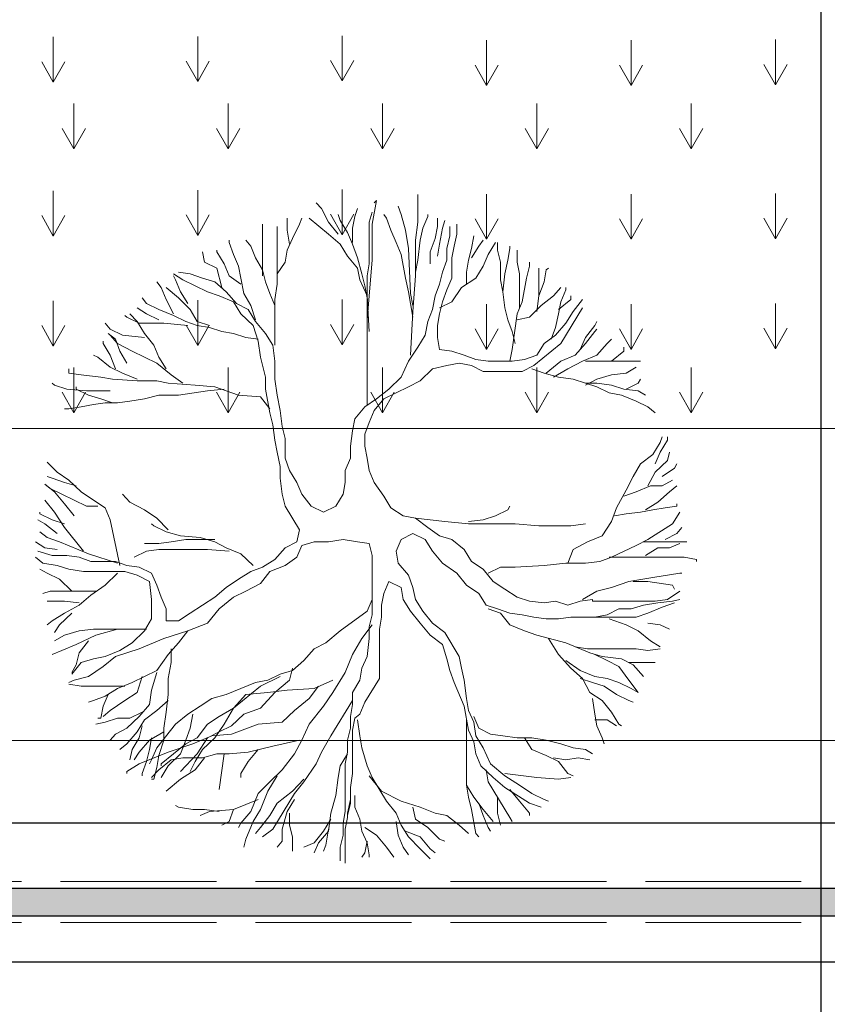
# Model space of a CAD drawing. Units: millimetres. Extents: x 595116 to 630915, y 909473 to 920225.
# Tile 42 of 134: x 629682 to 629744, y 919141 to 919216. Entities that reach past the tile are written whole.
import ezdxf

# ---------------------------------------------------------------- set-up
doc = ezdxf.new("R2010")
doc.units = ezdxf.units.MM
doc.linetypes.add('ACAD_ISO02W100', pattern=[15, 12, -3])
for name, color, linetype, lineweight in [('C-PROP', 7, 'Continuous', 25), ('C-PROP-REF', 240, 'ACAD_ISO02W100', 13), ('Dimension', 3, 'Continuous', 18), ('L-PLNT', 85, 'Continuous', 13)]:
    doc.layers.add(name, color=color, linetype=linetype, lineweight=lineweight)
doc.styles.get("Standard").update_dxf_attribs({"font": 'arial.ttf'})
doc.dimstyles.new('ISO-25', dxfattribs={"dimtxt": 9, "dimasz": 6, "dimexe": 1.25, "dimexo": 0.625, "dimtad": 1, "dimlunit": 4, "dimtxsty": 'Standard', "dimcen": 2.5, "dimadec": 0, "dimazin": 0, "dimtfac": 1, "dimtmove": 0, "dimatfit": 3, "dimfxl": 1, "dimarcsym": 0})

# ---------------------------------------------------------------- blocks, each defined once
blk = doc.blocks.new('A$C143125F4')
for p, q in [((2.1554, 4.9368), (2.1171, 4.9816)), ((2.5383, 4.8203), (2.5711, 4.9995)), ((2.5711, 4.9995), (2.5547, 4.9816)), ((2.883, 4.8338), (2.883, 5.0443)), ((2.2101, 4.8338), (2.1554, 4.9368)), ((2.407, 4.8786), (2.4289, 4.9368)), ((2.5164, 4.8338), (2.5383, 4.9099)), ((2.7571, 4.892), (2.7353, 4.9547)), ((1.8983, 4.7755), (1.8983, 4.8651)), ((1.9913, 4.8203), (2.0077, 4.8651)), ((2.2101, 4.7442), (2.0624, 4.8651)), ((2.2812, 4.7442), (2.2101, 4.8338)), ((2.2976, 4.8472), (2.2812, 4.892)), ((2.3523, 4.7576), (2.2976, 4.8472)), ((2.3906, 4.789), (2.407, 4.8786)), ((2.5164, 4.5202), (2.5164, 4.8338)), ((2.6477, 4.8651), (2.6259, 4.892)), ((2.6806, 4.7755), (2.6477, 4.8651)), ((2.79, 4.7755), (2.7571, 4.892)), ((2.8666, 4.6994), (2.883, 4.8338)), ((2.9213, 4.789), (2.9596, 4.8786)), ((2.9596, 4.8786), (2.9596, 4.892)), ((3.0307, 4.8024), (3.0307, 4.8651)), ((3.069, 4.789), (3.0854, 4.8472)), ((1.7123, 4.4306), (1.7123, 4.8203)), ((1.8217, 4.3679), (1.8217, 4.8024)), ((1.9147, 4.668), (1.8983, 4.7755)), ((1.9366, 4.7128), (1.9913, 4.8203)), ((2.3906, 4.668), (2.3523, 4.7576)), ((2.3906, 4.6814), (2.3906, 4.789)), ((2.5383, 4.5471), (2.5383, 4.8203)), ((2.7189, 4.6814), (2.6806, 4.7755)), ((2.8119, 4.6367), (2.79, 4.7755)), ((2.8994, 4.6994), (2.9213, 4.789)), ((3.0143, 4.7128), (3.0307, 4.8024)), ((3.0471, 4.668), (3.069, 4.789)), ((3.1237, 4.7307), (3.1237, 4.8024)), ((3.1784, 4.7442), (3.1784, 4.8203)), ((1.4606, 4.6814), (1.4606, 4.6994)), ((1.4935, 4.5919), (1.4606, 4.6814)), ((1.6247, 4.6546), (1.5865, 4.6994)), ((1.8983, 4.6232), (1.9366, 4.7128)), ((2.2976, 4.668), (2.2101, 4.7442)), ((2.7571, 4.5919), (2.7189, 4.6814)), ((2.8666, 4.4306), (2.8666, 4.6994)), ((2.883, 4.5471), (2.8994, 4.6994)), ((2.976, 4.6098), (3.0143, 4.7128)), ((3.1018, 4.6367), (3.1237, 4.7307)), ((3.1565, 4.6546), (3.1784, 4.7442)), ((3.2878, 4.6367), (3.3042, 4.7307)), ((3.3425, 4.6546), (3.3753, 4.6994)), ((3.4136, 4.5919), (3.4683, 4.6814)), ((3.4847, 4.6232), (3.4847, 4.6814)), ((1.2746, 4.5336), (1.2582, 4.6098)), ((1.3676, 4.6098), (1.3676, 4.6232)), ((1.4223, 4.5202), (1.3676, 4.6098)), ((1.6576, 4.565), (1.6247, 4.6546)), ((1.8819, 4.5336), (1.8983, 4.6232)), ((2.3523, 4.5784), (2.2976, 4.668)), ((2.4289, 4.565), (2.3906, 4.668)), ((2.8283, 4.2962), (2.8119, 4.6367)), ((2.976, 4.5202), (2.976, 4.6098)), ((3.0307, 4.5784), (3.0471, 4.668)), ((3.1018, 4.5471), (3.1018, 4.6367)), ((3.1401, 4.565), (3.1565, 4.6546)), ((3.2659, 4.5471), (3.2878, 4.6367)), ((3.2878, 4.565), (3.3425, 4.6546)), ((3.5066, 4.5336), (3.4847, 4.6232)), ((3.5613, 4.5471), (3.5777, 4.6367)), ((3.5777, 4.6367), (3.5777, 4.6546)), ((3.6324, 4.5336), (3.6324, 4.6232)), ((1.3676, 4.4888), (1.2746, 4.5336)), ((1.5317, 4.5023), (1.4935, 4.5919)), ((1.7123, 4.4754), (1.6576, 4.565)), ((1.8217, 4.444), (1.8819, 4.5336)), ((2.4289, 4.4888), (2.3523, 4.5784)), ((2.4617, 4.444), (2.4289, 4.565)), ((2.5, 4.0991), (2.5383, 4.5471)), ((2.79, 4.4127), (2.7571, 4.5919)), ((2.8666, 4.4575), (2.883, 4.5471)), ((3.069, 4.4575), (3.1018, 4.5471)), ((3.1401, 4.4127), (3.1401, 4.565)), ((3.2495, 4.4575), (3.2659, 4.5471)), ((3.3753, 4.5023), (3.4136, 4.5919)), ((3.5066, 4.3992), (3.5066, 4.5336)), ((3.5394, 4.444), (3.5613, 4.5471)), ((3.6488, 4.444), (3.6324, 4.5336)), ((3.7254, 4.5023), (3.7254, 4.5336)), ((1.0777, 4.4575), (1.1652, 4.444)), ((1.4059, 4.341), (1.3676, 4.4888)), ((1.4606, 4.4306), (1.4223, 4.5202)), ((1.5482, 4.4127), (1.5317, 4.5023)), ((1.7342, 4.3858), (1.7123, 4.4754)), ((2.4453, 4.3992), (2.4289, 4.4888)), ((2.5, 4.4306), (2.5164, 4.5202)), ((3.0471, 4.3679), (3.069, 4.4575)), ((3.2495, 4.3679), (3.2495, 4.4575)), ((3.3206, 4.4127), (3.3753, 4.5023)), ((3.7035, 4.4127), (3.7254, 4.5023)), ((3.7965, 4.2783), (3.7965, 4.4888)), ((3.8348, 4.3858), (3.8512, 4.4754)), ((3.8512, 4.4754), (3.8677, 4.4888)), ((0.9464, 4.341), (0.9136, 4.3858)), ((1.1105, 4.3992), (1.0394, 4.444)), ((1.0558, 4.3992), (1.0394, 4.4306)), ((1.0941, 4.3096), (1.0558, 4.3992)), ((1.2965, 4.3096), (1.1105, 4.3992)), ((1.1652, 4.444), (1.2582, 4.4127)), ((1.2582, 4.4127), (1.3512, 4.3858)), ((1.3512, 4.3858), (1.4387, 4.3096)), ((1.5482, 4.3679), (1.4606, 4.4306)), ((1.57, 4.2962), (1.5482, 4.4127)), ((1.767, 4.2962), (1.7342, 4.3858)), ((2.5, 4.2783), (2.4453, 4.3992)), ((2.4836, 4.3544), (2.4617, 4.444)), ((2.5, 3.4584), (2.5, 4.4306)), ((2.8119, 4.3096), (2.79, 4.4127)), ((2.8447, 4.1618), (2.8666, 4.4306)), ((3.1018, 4.3231), (3.1401, 4.4127)), ((3.2112, 4.341), (3.3206, 4.4127)), ((3.523, 4.3096), (3.5066, 4.3992)), ((3.523, 4.3096), (3.5394, 4.444)), ((3.6488, 4.1887), (3.6488, 4.444)), ((3.6707, 4.2335), (3.7035, 4.4127)), ((3.7965, 4.2783), (3.8348, 4.3858)), ((0.9847, 4.2514), (0.9464, 4.341)), ((1.0777, 4.2648), (0.9847, 4.341)), ((1.1488, 4.22), (1.0941, 4.3096)), ((1.384, 4.2783), (1.2965, 4.3096)), ((1.4387, 4.3096), (1.5153, 4.22)), ((1.8053, 4.2514), (1.8217, 4.3679)), ((2.5, 4.2648), (2.4836, 4.3544)), ((2.8283, 4.22), (2.8119, 4.3096)), ((3.0143, 4.2783), (3.0471, 4.3679)), ((3.069, 4.2335), (3.1018, 4.3231)), ((3.1401, 4.2335), (3.2112, 4.341)), ((3.5394, 4.1887), (3.523, 4.3096)), ((3.906, 4.2783), (3.9607, 4.341)), ((3.9607, 4.2335), (3.999, 4.3231)), ((3.999, 4.3231), (3.999, 4.341)), ((0.837, 4.22), (0.8042, 4.2648)), ((1.0394, 4.1439), (0.9847, 4.2514)), ((1.1652, 4.1752), (1.0777, 4.2648)), ((1.4935, 4.2335), (1.384, 4.2783)), ((1.6247, 4.2066), (1.57, 4.2962)), ((1.8053, 4.2066), (1.767, 4.2962)), ((1.8053, 3.9064), (1.8053, 4.2514)), ((2.5164, 4.0095), (2.5, 4.2783)), ((2.8447, 4.2066), (2.8283, 4.2962)), ((2.9924, 4.1752), (3.0143, 4.2783)), ((3.7801, 4.1618), (3.7965, 4.2783)), ((3.813, 4.2066), (3.906, 4.2783)), ((3.9442, 4.1752), (4.0372, 4.2514)), ((4.0372, 4.2514), (4.0372, 4.2783)), ((4.1248, 4.2514), (4.0537, 4.1618)), ((0.837, 4.1439), (0.7659, 4.1887)), ((0.93, 4.1752), (0.837, 4.22)), ((1.0394, 4.1304), (0.93, 4.1752)), ((1.2199, 4.0856), (1.1652, 4.1752)), ((1.5482, 4.1439), (1.4935, 4.2335)), ((1.5153, 4.22), (1.6029, 4.1752)), ((1.6029, 4.1752), (1.6576, 4.0856)), ((1.6576, 4.0991), (1.6247, 4.2066)), ((2.8447, 4.117), (2.8283, 4.22)), ((2.8283, 3.8303), (2.8447, 4.1618)), ((2.9596, 4.0856), (2.9924, 4.1752)), ((3.0471, 4.1887), (3.1401, 4.2335)), ((3.0471, 4.1439), (3.069, 4.2335)), ((3.5613, 4.0991), (3.5394, 4.1887)), ((3.6324, 4.1439), (3.6707, 4.2335)), ((3.7254, 4.117), (3.813, 4.2066)), ((3.9442, 4.1439), (3.9607, 4.2335)), ((3.9607, 3.9199), (4.1248, 4.1887)), ((4.0537, 4.1618), (3.999, 4.0722)), ((0.6893, 4.117), (0.6729, 4.1304)), ((0.7823, 4.0722), (0.6893, 4.117)), ((0.7659, 4.0856), (0.7112, 4.1439)), ((0.8206, 3.996), (0.7659, 4.0856)), ((0.93, 4.0991), (0.837, 4.1439)), ((1.1324, 4.0856), (1.0394, 4.1304)), ((1.2199, 4.0543), (1.1324, 4.0856)), ((1.3129, 4.0543), (1.2199, 4.0856)), ((1.6412, 4.0543), (1.5482, 4.1439)), ((1.6576, 4.0856), (1.7342, 3.996)), ((2.5, 3.996), (2.5, 4.0991)), ((2.9377, 3.9826), (2.9596, 4.0856)), ((3.0307, 4.0543), (3.0471, 4.1439)), ((3.5941, 4.0095), (3.5613, 4.0991)), ((3.5941, 3.8751), (3.6324, 4.1439)), ((3.6324, 4.0991), (3.7254, 4.117)), ((3.9224, 4.0408), (3.9442, 4.1439)), ((4.2178, 4.0543), (4.2342, 4.0856)), ((0.5635, 4.0274), (0.5252, 4.0722)), ((0.6565, 3.9826), (0.5635, 4.0274)), ((0.9683, 4.0722), (0.7823, 4.0722)), ((1.1488, 4.0543), (0.9683, 4.0722)), ((1.3129, 4.0408), (1.2199, 4.0543)), ((1.4059, 4.0095), (1.3129, 4.0408)), ((1.6795, 3.9378), (1.6412, 4.0543)), ((3.0307, 3.9647), (3.0307, 4.0543)), ((3.8895, 3.9512), (3.9224, 4.0408)), ((3.999, 4.0722), (3.9224, 3.9826)), ((4.1467, 3.9647), (4.2178, 4.0543)), ((4.2178, 4.0095), (4.2342, 4.0274)), ((0.5088, 3.9199), (0.5088, 3.9378)), ((0.6018, 3.9512), (0.5471, 3.996)), ((0.6182, 3.9199), (0.5635, 3.9826)), ((0.6346, 3.8616), (0.6018, 3.9512)), ((0.8206, 3.9647), (0.6565, 3.9826)), ((0.8917, 3.9064), (0.8206, 3.996)), ((1.4935, 3.996), (1.4059, 4.0095)), ((1.5865, 3.9647), (1.4935, 3.996)), ((1.6795, 3.9512), (1.5865, 3.9647)), ((1.6959, 3.8168), (1.6795, 3.9378)), ((1.7342, 3.996), (1.7889, 3.9064)), ((2.883, 3.893), (2.9377, 3.9826)), ((3.0471, 3.8751), (3.0307, 3.9647)), ((3.616, 3.9199), (3.5941, 4.0095)), ((3.9224, 3.9826), (3.8348, 3.9199)), ((4.1084, 3.8751), (4.1467, 3.9647)), ((4.1467, 3.9199), (4.2178, 4.0095)), ((4.3108, 3.9199), (4.3436, 3.9512)), ((0.5635, 3.8303), (0.5088, 3.9199)), ((0.7276, 3.8616), (0.6182, 3.9199)), ((0.93, 3.8168), (0.8917, 3.9064)), ((1.7889, 3.9064), (1.8053, 3.7855)), ((2.8119, 3.7855), (2.883, 3.893)), ((3.1401, 3.8616), (3.0471, 3.8751)), ((3.5777, 3.7855), (3.5941, 3.8751)), ((3.7583, 3.7541), (3.9607, 3.9199)), ((3.8348, 3.9199), (3.7801, 3.8303)), ((4.0701, 3.8303), (4.1467, 3.9199)), ((4.2342, 3.8303), (4.3108, 3.9199)), ((4.4366, 3.8616), (4.4366, 3.893)), ((0.4705, 3.8168), (0.4376, 3.8303)), ((0.5635, 3.7407), (0.4705, 3.8168)), ((0.6018, 3.7272), (0.5635, 3.8303)), ((0.6893, 3.772), (0.6346, 3.8616)), ((0.9136, 3.772), (0.7276, 3.8616)), ((0.9847, 3.7272), (0.93, 3.8168)), ((1.7342, 3.6645), (1.6959, 3.8168)), ((3.2331, 3.8303), (3.1401, 3.8616)), ((3.3206, 3.7989), (3.2331, 3.8303)), ((3.4136, 3.7855), (3.3206, 3.7989)), ((3.6871, 3.7989), (3.5941, 3.7855)), ((3.7801, 3.8303), (3.6871, 3.7989)), ((3.9607, 3.7855), (4.0701, 3.8303)), ((4.1248, 3.7855), (4.2342, 3.8303)), ((4.3436, 3.7855), (4.4366, 3.8616)), ((0.2516, 3.6959), (0.2516, 3.7272)), ((0.6565, 3.6959), (0.5635, 3.7407)), ((1.023, 3.6824), (0.9136, 3.772)), ((1.8053, 3.7855), (1.8053, 3.6511)), ((2.7571, 3.6645), (2.8119, 3.7855)), ((2.8994, 3.6376), (2.9924, 3.7272)), ((2.9924, 3.7272), (3.1018, 3.7541)), ((3.1018, 3.7541), (3.1948, 3.772)), ((3.1948, 3.772), (3.2878, 3.7541)), ((3.2878, 3.7541), (3.3753, 3.7093)), ((3.5941, 3.7855), (3.4136, 3.7855)), ((3.6707, 3.7093), (3.7583, 3.7541)), ((3.7418, 3.7272), (3.8348, 3.6959)), ((3.8512, 3.6959), (3.9607, 3.7855)), ((3.906, 3.6645), (4.0154, 3.7272)), ((4.0154, 3.7272), (4.1248, 3.7855)), ((4.1467, 3.7855), (4.5624, 3.7855)), ((4.453, 3.6959), (4.5296, 3.7407)), ((0.3446, 3.6824), (0.2516, 3.6959)), ((0.4923, 3.6645), (0.3446, 3.6824)), ((0.5799, 3.6511), (0.4923, 3.6645)), ((0.7659, 3.6376), (0.5799, 3.6511)), ((0.7659, 3.6511), (0.6565, 3.6959)), ((1.1105, 3.6197), (1.023, 3.6824)), ((1.7342, 3.5749), (1.7342, 3.6645)), ((1.8053, 3.6511), (1.8217, 3.5301)), ((2.6641, 3.5749), (2.7571, 3.6645)), ((3.3753, 3.7093), (3.6707, 3.7093)), ((3.8348, 3.6959), (3.9442, 3.6645)), ((3.9442, 3.6645), (4.0537, 3.6511)), ((4.0537, 3.6511), (4.1467, 3.6197)), ((4.1467, 3.6063), (4.2342, 3.6511)), ((4.2342, 3.6511), (4.3436, 3.6824)), ((4.3436, 3.6824), (4.453, 3.6959)), ((4.546, 3.6197), (4.5624, 3.6511)), ((0.1422, 3.6063), (0.1258, 3.6197)), ((0.2352, 3.5749), (0.1422, 3.6063)), ((0.3829, 3.5615), (0.2352, 3.5749)), ((0.3063, 3.5749), (0.3063, 3.5928)), ((0.3993, 3.5301), (0.3063, 3.5749)), ((0.9136, 3.6376), (0.7659, 3.6376)), ((1.0011, 3.6197), (0.9136, 3.6376)), ((1.2035, 3.6063), (1.0011, 3.6197)), ((1.3512, 3.5928), (1.2035, 3.6063)), ((1.4223, 3.5749), (1.2965, 3.5615)), ((1.5317, 3.5301), (1.3512, 3.5928)), ((1.767, 3.3957), (1.7342, 3.5749)), ((2.5711, 3.5032), (2.6641, 3.5749)), ((2.6259, 3.5032), (2.8119, 3.5928)), ((2.8119, 3.5928), (2.8994, 3.6376)), ((4.1467, 3.6197), (4.2342, 3.5928)), ((4.1467, 3.6197), (4.2342, 3.6197)), ((4.2342, 3.6197), (4.3436, 3.6063)), ((4.2342, 3.5928), (4.3272, 3.548)), ((4.3436, 3.6063), (4.4366, 3.5749)), ((4.4366, 3.5749), (4.546, 3.5615)), ((4.453, 3.5749), (4.546, 3.6197)), ((0.5635, 3.5615), (0.3829, 3.5615)), ((0.4923, 3.5032), (0.3993, 3.5301)), ((0.5799, 3.4719), (0.4923, 3.5032)), ((0.8206, 3.5032), (0.7112, 3.4853)), ((0.93, 3.5301), (0.8206, 3.5032)), ((1.0777, 3.5301), (0.93, 3.5301)), ((1.2965, 3.5615), (1.0777, 3.5301)), ((1.6959, 3.5167), (1.5317, 3.5301)), ((1.767, 3.4271), (1.6959, 3.5167)), ((1.8217, 3.5301), (1.8436, 3.4136)), ((2.4836, 3.4405), (2.5711, 3.5032)), ((2.5547, 3.4136), (2.6259, 3.5032)), ((4.3272, 3.548), (4.4202, 3.5301)), ((4.4202, 3.5301), (4.5296, 3.4853)), ((4.546, 3.5615), (4.6007, 3.5301)), ((0.2516, 3.4271), (0.2188, 3.4271)), ((0.3446, 3.4405), (0.2516, 3.4271)), ((0.4376, 3.4584), (0.3446, 3.4405)), ((0.5252, 3.4719), (0.4376, 3.4584)), ((0.6182, 3.4719), (0.5252, 3.4719)), ((0.7112, 3.4853), (0.6182, 3.4719)), ((2.407, 3.3509), (2.4836, 3.4405)), ((4.5296, 3.4853), (4.6171, 3.4405)), ((4.6171, 3.4405), (4.6718, 3.3957)), ((1.7889, 3.3061), (1.767, 3.3957)), ((1.8436, 3.4136), (1.86, 3.2927)), ((2.3906, 3.2613), (2.407, 3.3509)), ((2.5164, 3.3241), (2.5547, 3.4136)), ((1.8053, 3.1897), (1.7889, 3.3061)), ((1.86, 3.2927), (1.8819, 3.2031)), ((2.4836, 3.2345), (2.5164, 3.3241)), ((1.8819, 3.2031), (1.8819, 3.0553)), ((2.3742, 3.1449), (2.3906, 3.2613)), ((2.4836, 3.1449), (2.4836, 3.2345)), ((4.7101, 3.1717), (4.7265, 3.2165)), ((4.7648, 3.1897), (4.7648, 3.2165)), ((1.8217, 3.1001), (1.8053, 3.1897)), ((2.3742, 3.0553), (2.3742, 3.1449)), ((2.5, 3.0553), (2.4836, 3.1449)), ((4.6554, 3.0821), (4.7101, 3.1717)), ((4.7101, 3.1001), (4.7648, 3.1897)), ((1.8436, 2.9925), (1.8217, 3.1001)), ((1.8819, 3.0553), (1.9147, 2.9612)), ((2.3359, 2.9612), (2.3742, 3.0553)), ((2.5164, 2.9612), (2.5, 3.0553)), ((4.5624, 3.0105), (4.6554, 3.0821)), ((4.6718, 3.0105), (4.7101, 3.1001)), ((4.7648, 3.0373), (4.7812, 3.1001)), ((0.1641, 2.9477), (0.0875, 3.0239)), ((1.8436, 2.9029), (1.8436, 2.9925)), ((4.5077, 2.9164), (4.5624, 3.0105)), ((4.6718, 2.9477), (4.7648, 3.0373)), ((4.7265, 2.9164), (4.8195, 2.9791)), ((4.8195, 2.9791), (4.8359, 3.0105)), ((0.1258, 2.9029), (0.0875, 2.9164)), ((0.2188, 2.8716), (0.1258, 2.9029)), ((0.2516, 2.8895), (0.1641, 2.9477)), ((1.86, 2.782), (1.8436, 2.9029)), ((1.9147, 2.9612), (1.9694, 2.8716)), ((2.3359, 2.8716), (2.3359, 2.9612)), ((2.5547, 2.8716), (2.5164, 2.9612)), ((4.453, 2.8133), (4.5077, 2.9164)), ((4.6171, 2.8447), (4.6718, 2.9477)), ((0.1422, 2.7999), (0.0711, 2.8581)), ((0.1094, 2.8268), (0.0711, 2.8581)), ((0.1969, 2.782), (0.1094, 2.8268)), ((0.3063, 2.8447), (0.2188, 2.8716)), ((0.3446, 2.7999), (0.2516, 2.8895)), ((1.9694, 2.8716), (2.0077, 2.782)), ((2.3195, 2.782), (2.3359, 2.8716)), ((2.6259, 2.7686), (2.5547, 2.8716)), ((4.5296, 2.7999), (4.639, 2.8447)), ((4.639, 2.8447), (4.7265, 2.8447)), ((4.7265, 2.8447), (4.8031, 2.8895)), ((4.7812, 2.7999), (4.8359, 2.8447)), ((0.2188, 2.7103), (0.1422, 2.7999)), ((0.3829, 2.6924), (0.1969, 2.782)), ((0.4376, 2.7372), (0.3446, 2.7999)), ((0.7112, 2.7238), (0.6565, 2.782)), ((1.8819, 2.6924), (1.86, 2.782)), ((2.0077, 2.782), (2.0788, 2.6924)), ((2.2648, 2.6924), (2.3195, 2.782)), ((2.6806, 2.679), (2.6259, 2.7686)), ((4.3819, 2.679), (4.453, 2.8133)), ((4.4366, 2.7686), (4.5296, 2.7999)), ((4.6937, 2.7238), (4.7812, 2.7999)), ((0.1422, 2.6476), (0.0711, 2.7372)), ((0.2899, 2.6207), (0.2188, 2.7103)), ((0.4705, 2.6924), (0.3829, 2.6924)), ((0.5252, 2.679), (0.4376, 2.7372)), ((0.5635, 2.5894), (0.5252, 2.679)), ((0.8206, 2.6655), (0.7112, 2.7238)), ((1.9913, 2.5132), (1.8819, 2.6924)), ((2.0788, 2.6924), (2.1718, 2.6476)), ((2.1718, 2.6476), (2.2648, 2.6924)), ((2.7736, 2.6207), (2.6806, 2.679)), ((3.5613, 2.6655), (3.5777, 2.6924)), ((4.3436, 2.5759), (4.3819, 2.679)), ((4.6007, 2.6655), (4.6937, 2.7238)), ((4.6554, 2.6655), (4.7484, 2.679)), ((4.7484, 2.679), (4.8359, 2.6924)), ((4.8359, 2.6924), (4.8359, 2.7103)), ((0.0328, 2.6342), (0.0328, 2.6476)), ((0.1258, 2.5894), (0.0328, 2.6342)), ((0.2188, 2.5311), (0.1422, 2.6476)), ((0.9136, 2.6028), (0.8206, 2.6655)), ((1.0011, 2.5132), (0.9136, 2.6028)), ((2.8666, 2.6028), (2.7736, 2.6207)), ((2.8666, 2.6028), (3.0854, 2.5759)), ((2.9596, 2.5311), (2.8666, 2.6028)), ((3.3753, 2.5894), (3.4683, 2.6207)), ((3.4683, 2.6207), (3.5613, 2.6655)), ((4.3655, 2.6207), (4.453, 2.6342)), ((4.453, 2.6342), (4.5624, 2.6476)), ((4.5624, 2.6476), (4.6554, 2.6655)), ((4.8031, 2.558), (4.8578, 2.6476)), ((0.0711, 2.558), (0.0164, 2.5894)), ((0.1641, 2.4863), (0.0711, 2.558)), ((0.2188, 2.558), (0.1258, 2.5894)), ((0.3611, 2.3519), (0.2188, 2.5311)), ((0.6346, 2.2444), (0.5635, 2.5894)), ((0.8917, 2.5446), (0.8753, 2.558)), ((0.9847, 2.4998), (0.8917, 2.5446)), ((3.0471, 2.4684), (2.9596, 2.5311)), ((3.0854, 2.5759), (3.2659, 2.558)), ((3.2659, 2.5759), (3.3753, 2.5894)), ((3.2659, 2.558), (3.616, 2.558)), ((3.616, 2.558), (3.7965, 2.5446)), ((3.7965, 2.5446), (4.0372, 2.5446)), ((4.0372, 2.5446), (4.1467, 2.558)), ((4.2725, 2.4684), (4.3436, 2.5759)), ((4.6171, 2.4415), (4.8031, 2.558)), ((4.8359, 2.4863), (4.8742, 2.5311)), ((0.0875, 2.455), (0.0328, 2.4998)), ((0.1805, 2.4236), (0.0875, 2.455)), ((1.0941, 2.4684), (0.9847, 2.4998)), ((1.2418, 2.455), (1.0941, 2.4684)), ((1.3512, 2.4236), (1.2418, 2.455)), ((1.9694, 2.4236), (1.9913, 2.5132)), ((2.8447, 2.4863), (2.7571, 2.4415)), ((2.9377, 2.4415), (2.8447, 2.4863)), ((3.1401, 2.4415), (3.0471, 2.4684)), ((4.1631, 2.4236), (4.2725, 2.4684)), ((4.7484, 2.4415), (4.8359, 2.4863)), ((0.0711, 2.3788), (0, 2.4236)), ((0.1641, 2.3654), (0.0711, 2.3788)), ((0.3993, 2.334), (0.1805, 2.4236)), ((0.93, 2.4102), (0.8206, 2.4102)), ((1.023, 2.4236), (0.93, 2.4102)), ((1.1324, 2.4415), (1.023, 2.4236)), ((1.3512, 2.4415), (1.1324, 2.4415)), ((1.4387, 2.3788), (1.3512, 2.4236)), ((1.5482, 2.334), (1.4387, 2.3788)), ((1.8053, 2.2892), (1.8819, 2.3788)), ((1.8819, 2.3788), (1.9694, 2.4236)), ((2.0077, 2.3967), (1.9694, 2.3071)), ((2.1007, 2.4236), (2.0077, 2.3967)), ((2.2101, 2.4236), (2.1007, 2.4236)), ((2.3195, 2.4415), (2.2101, 2.4236)), ((2.4289, 2.4236), (2.3195, 2.4415)), ((2.5164, 2.4102), (2.4289, 2.4236)), ((2.5383, 2.3206), (2.5164, 2.4102)), ((2.7571, 2.4415), (2.7189, 2.3519)), ((2.9924, 2.3519), (2.9377, 2.4415)), ((3.2331, 2.3654), (3.1401, 2.4415)), ((4.0537, 2.3654), (4.1631, 2.4236)), ((4.3436, 2.3071), (4.5296, 2.3967)), ((4.5296, 2.3967), (4.6171, 2.4415)), ((4.5843, 2.4236), (4.9125, 2.4236)), ((4.6007, 2.3206), (4.6937, 2.3788)), ((4.6937, 2.3788), (4.7812, 2.3788)), ((4.7812, 2.3788), (4.8578, 2.4102)), ((0.0547, 2.2623), (0, 2.3071)), ((0.0164, 2.3519), (0.1258, 2.3206)), ((0.1258, 2.3206), (0.2352, 2.3206)), ((0.2352, 2.3206), (0.3282, 2.3071)), ((0.3282, 2.3071), (0.4158, 2.2758)), ((0.6182, 2.2623), (0.3993, 2.334)), ((0.837, 2.3519), (0.744, 2.3071)), ((0.93, 2.3654), (0.837, 2.3519)), ((1.2965, 2.3654), (0.93, 2.3654)), ((1.4606, 2.3519), (1.2965, 2.3654)), ((1.6412, 2.2444), (1.5482, 2.334)), ((1.9694, 2.3071), (1.8819, 2.2444)), ((2.5383, 1.8726), (2.5383, 2.3206)), ((2.7189, 2.3519), (2.7353, 2.2623)), ((3.069, 2.2623), (2.9924, 2.3519)), ((3.2878, 2.2758), (3.2331, 2.3654)), ((4.0154, 2.2623), (4.0537, 2.3654)), ((4.2561, 2.2758), (4.3436, 2.3071)), ((4.3272, 2.3071), (4.8906, 2.3071)), ((4.8906, 2.3071), (4.9836, 2.2892)), ((0.1641, 2.2444), (0.0547, 2.2623)), ((0.2516, 2.2175), (0.1641, 2.2444)), ((0.4158, 2.2758), (0.6018, 2.2758)), ((0.6018, 2.2758), (0.6893, 2.2444)), ((0.6893, 2.2444), (0.7823, 2.231)), ((0.7823, 2.231), (0.8753, 2.1862)), ((1.6247, 2.1996), (1.7123, 2.231)), ((1.7123, 2.231), (1.8053, 2.2892)), ((1.8819, 2.2444), (1.767, 2.1996)), ((2.7353, 2.2623), (2.8119, 2.1727)), ((3.1784, 2.1862), (3.069, 2.2623)), ((3.3753, 2.2175), (3.2878, 2.2758)), ((3.4136, 2.1862), (3.5066, 2.231)), ((3.5066, 2.231), (3.616, 2.231)), ((3.616, 2.231), (3.8348, 2.2444)), ((3.8348, 2.2444), (3.999, 2.2623)), ((3.999, 2.2623), (4.1467, 2.2623)), ((4.1467, 2.2623), (4.2561, 2.2758)), ((4.9836, 2.2892), (4.9836, 2.2758)), ((0.0875, 2.1862), (0.0328, 2.2175)), ((0.1805, 2.1414), (0.0875, 2.1862)), ((0.3611, 2.1996), (0.2516, 2.2175)), ((0.6729, 2.1996), (0.3611, 2.1996)), ((0.6182, 2.1862), (0.5252, 2.0966)), ((0.7659, 2.1727), (0.6729, 2.1996)), ((0.8589, 2.1235), (0.7659, 2.1727)), ((0.8753, 2.1862), (0.9136, 2.0966)), ((1.5317, 2.1414), (1.6247, 2.1996)), ((1.767, 2.1996), (1.6959, 2.11)), ((2.8119, 2.1727), (2.8447, 2.0787)), ((3.2495, 2.0966), (3.1784, 2.1862)), ((3.4519, 2.1235), (3.3753, 2.2175)), ((4.4749, 2.1235), (4.6554, 2.1548)), ((4.6554, 2.1548), (4.8578, 2.1862)), ((4.8578, 2.1862), (4.8742, 2.1862)), ((0.2735, 2.0518), (0.1805, 2.1414)), ((0.5252, 2.0966), (0.4158, 2.0204)), ((0.8753, 1.9891), (0.8589, 2.1235)), ((0.9136, 2.0966), (0.9464, 2.007)), ((1.4387, 2.0787), (1.5317, 2.1414)), ((1.6959, 2.11), (1.5865, 2.0518)), ((2.6641, 2.1235), (2.6259, 2.0339)), ((2.7571, 2.0787), (2.6641, 2.1235)), ((3.3425, 2.0339), (3.2495, 2.0966)), ((3.5394, 2.0652), (3.4519, 2.1235)), ((4.3436, 2.0787), (4.4749, 2.1235)), ((4.5077, 2.1235), (4.6171, 2.1235)), ((4.6171, 2.1235), (4.8031, 2.0966)), ((4.8031, 2.0966), (4.8195, 2.0652)), ((0.1094, 2.0518), (0.0547, 2.0339)), ((0.4541, 2.0518), (0.1094, 2.0518)), ((0.4158, 2.0204), (0.3282, 1.9443)), ((0.9464, 2.007), (0.9847, 1.9174)), ((1.2582, 1.9443), (1.3512, 2.007)), ((1.3512, 2.007), (1.4387, 2.0787)), ((1.4935, 2.007), (1.384, 1.9174)), ((1.5865, 2.0518), (1.4935, 2.007)), ((2.6259, 2.0339), (2.6094, 1.9443)), ((2.7736, 1.9891), (2.7571, 2.0787)), ((2.8447, 2.0787), (2.8666, 1.9891)), ((3.3972, 1.9443), (3.3425, 2.0339)), ((3.6324, 2.007), (3.5394, 2.0652)), ((3.7254, 1.9756), (3.6324, 2.007)), ((4.1248, 1.9891), (4.2342, 2.0518)), ((4.2342, 2.0518), (4.3436, 2.0787)), ((4.8578, 2.0518), (4.7648, 1.9891)), ((0.2188, 1.9756), (0.0875, 1.9756)), ((0.3282, 1.9622), (0.2188, 1.9756)), ((0.3282, 1.9443), (0.2188, 1.886)), ((0.8753, 1.8412), (0.8753, 1.9891)), ((1.1652, 1.886), (1.2582, 1.9443)), ((2.5383, 1.9891), (2.5, 1.8995)), ((2.6094, 1.9443), (2.6094, 1.8547)), ((2.8283, 1.8995), (2.7736, 1.9891)), ((2.8666, 1.9891), (2.9213, 1.8995)), ((3.4847, 1.9174), (3.3972, 1.9443)), ((3.8348, 1.9622), (3.7254, 1.9756)), ((3.9224, 1.9756), (3.8348, 1.9622)), ((4.0154, 1.9443), (3.9224, 1.9756)), ((4.1084, 1.9756), (4.0154, 1.9443)), ((4.2014, 1.9891), (4.1084, 1.9756)), ((4.2014, 1.9756), (4.2014, 1.9891)), ((4.6718, 1.9756), (4.2014, 1.9756)), ((4.4913, 1.9174), (4.5843, 1.9443)), ((4.5843, 1.9443), (4.6937, 1.9622)), ((4.7648, 1.9891), (4.6718, 1.9756)), ((4.6937, 1.9622), (4.8031, 1.9756)), ((4.8195, 1.9622), (4.7265, 1.9308)), ((4.8031, 1.9756), (4.8578, 1.9891)), ((0.2188, 1.886), (0.1258, 1.8278)), ((0.2735, 1.886), (0.1805, 1.7964)), ((0.9847, 1.9174), (0.9847, 1.8278)), ((1.0777, 1.8278), (1.1652, 1.886)), ((1.384, 1.9174), (1.2965, 1.8099)), ((2.5, 1.8995), (2.2976, 1.7516)), ((2.5164, 1.783), (2.5383, 1.8726)), ((2.8994, 1.8099), (2.8283, 1.8995)), ((2.9213, 1.8995), (2.9924, 1.8099)), ((3.4136, 1.9174), (3.5066, 1.886)), ((3.5777, 1.886), (3.4847, 1.9174)), ((3.5066, 1.886), (3.5777, 1.7964)), ((3.6707, 1.8726), (3.5777, 1.886)), ((3.7583, 1.8547), (3.6707, 1.8726)), ((4.2178, 1.8547), (4.3108, 1.8726)), ((4.3108, 1.8726), (4.3983, 1.9174)), ((4.3983, 1.9174), (4.4913, 1.9174)), ((4.6171, 1.886), (4.5296, 1.8547)), ((4.7265, 1.9308), (4.6171, 1.886)), ((0.1258, 1.8278), (0.0875, 1.7964)), ((0.1805, 1.7964), (0.1422, 1.7382)), ((0.8206, 1.7516), (0.8753, 1.8412)), ((0.9847, 1.8278), (1.0777, 1.8278)), ((1.2965, 1.8099), (1.1488, 1.7516)), ((2.5383, 1.7964), (2.4617, 1.6934)), ((2.5164, 1.6934), (2.5164, 1.783)), ((2.6094, 1.8547), (2.593, 1.7651)), ((2.976, 1.7203), (2.8994, 1.8099)), ((2.9924, 1.8099), (3.0854, 1.7382)), ((3.5777, 1.7964), (3.6871, 1.7516)), ((3.8512, 1.8412), (3.7583, 1.8547)), ((3.9442, 1.8412), (3.8512, 1.8412)), ((4.0372, 1.8547), (3.9442, 1.8412)), ((4.1248, 1.8547), (4.0372, 1.8547)), ((4.5296, 1.8547), (4.1248, 1.8547)), ((4.3272, 1.8412), (4.453, 1.7964)), ((4.453, 1.7964), (4.546, 1.7516)), ((4.6171, 1.8099), (4.7101, 1.7964)), ((4.7101, 1.7964), (4.7812, 1.7651)), ((0.2188, 1.7203), (0.1422, 1.6755)), ((0.3282, 1.7516), (0.2188, 1.7203)), ((0.4541, 1.7203), (0.3063, 1.6486)), ((0.4376, 1.7651), (0.3282, 1.7516)), ((0.837, 1.7651), (0.4376, 1.7651)), ((0.6182, 1.7651), (0.4541, 1.7203)), ((0.7276, 1.662), (0.8206, 1.7516)), ((1.1488, 1.7516), (0.9683, 1.6934)), ((1.1488, 1.7516), (1.0777, 1.662)), ((2.2976, 1.7516), (2.1882, 1.662)), ((2.593, 1.7651), (2.593, 1.3932)), ((3.069, 1.6486), (2.976, 1.7203)), ((3.0854, 1.7382), (3.1948, 1.559)), ((3.6871, 1.7516), (3.7801, 1.7203)), ((3.7801, 1.7203), (3.999, 1.662)), ((4.546, 1.7516), (4.639, 1.6755)), ((0.3063, 1.6486), (0.1969, 1.6038)), ((0.3993, 1.6755), (0.3282, 1.5859)), ((0.6346, 1.6038), (0.7276, 1.662)), ((0.9683, 1.6934), (0.7823, 1.6172)), ((1.0777, 1.662), (1.0011, 1.5724)), ((2.1882, 1.662), (2.1007, 1.6172)), ((2.4617, 1.6934), (2.3906, 1.5724)), ((2.5, 1.559), (2.5164, 1.6934)), ((3.1018, 1.5411), (3.069, 1.6486)), ((3.8677, 1.6934), (3.9442, 1.5724)), ((3.999, 1.662), (4.1795, 1.5859)), ((4.639, 1.6755), (4.7101, 1.6307)), ((0.1969, 1.6038), (0.1258, 1.5724)), ((0.3282, 1.5859), (0.3063, 1.4963)), ((0.5252, 1.559), (0.6346, 1.6038)), ((0.7823, 1.6172), (0.6018, 1.559)), ((1.0011, 1.5724), (0.9136, 1.4515)), ((1.023, 1.6172), (1.023, 1.5142)), ((2.1007, 1.6172), (2.0241, 1.5276)), ((2.3906, 1.5724), (2.3359, 1.438)), ((3.9442, 1.5724), (4.0372, 1.4694)), ((4.0701, 1.6307), (4.1631, 1.6172)), ((4.1631, 1.6172), (4.5296, 1.6172)), ((4.1795, 1.5859), (4.2725, 1.559)), ((4.2178, 1.5724), (4.3108, 1.5276)), ((4.5296, 1.6172), (4.6171, 1.6038)), ((4.6171, 1.6038), (4.7101, 1.6172)), ((0.2735, 1.4246), (0.3446, 1.5142)), ((0.3063, 1.4963), (0.2735, 1.438)), ((0.3446, 1.5142), (0.4376, 1.5411)), ((0.4376, 1.5411), (0.5252, 1.559)), ((0.6018, 1.559), (0.5088, 1.4828)), ((1.023, 1.5142), (1.0011, 1.3932)), ((2.0241, 1.5276), (1.9366, 1.4515)), ((2.4617, 1.4694), (2.5, 1.559)), ((3.1237, 1.4515), (3.1018, 1.5411)), ((3.1948, 1.559), (3.2112, 1.4694)), ((3.999, 1.5276), (4.1084, 1.4515)), ((4.2725, 1.559), (4.4202, 1.5411)), ((4.3108, 1.5276), (4.3983, 1.4828)), ((4.4202, 1.5411), (4.5077, 1.4963)), ((4.4749, 1.5142), (4.6718, 1.5142)), ((4.5077, 1.4963), (4.5843, 1.4067)), ((0.5088, 1.4828), (0.3993, 1.4067)), ((0.9136, 1.4515), (0.7276, 1.3619)), ((0.9136, 1.438), (0.8753, 1.3036)), ((1.8436, 1.4246), (1.7506, 1.3798)), ((1.9366, 1.4515), (1.8436, 1.4246)), ((1.9366, 1.4694), (1.9147, 1.3798)), ((2.3359, 1.438), (2.2429, 1.2857)), ((2.4453, 1.3798), (2.4617, 1.4694)), ((3.1565, 1.3619), (3.1237, 1.4515)), ((3.2112, 1.4694), (3.2331, 1.3798)), ((4.0372, 1.4694), (4.1248, 1.3932)), ((4.1084, 1.4515), (4.2178, 1.4067)), ((4.3983, 1.4828), (4.4749, 1.3798)), ((0.2899, 1.3798), (0.2516, 1.3619)), ((0.3446, 1.335), (0.2516, 1.3484)), ((0.3993, 1.4067), (0.2899, 1.3798)), ((0.7276, 1.3619), (0.6182, 1.3171)), ((0.8042, 1.4067), (0.7659, 1.2857)), ((1.0011, 1.3932), (1.0011, 1.2723)), ((1.6576, 1.3619), (1.4387, 1.2723)), ((1.7506, 1.3798), (1.6576, 1.3619)), ((1.8436, 1.4067), (1.6959, 1.335)), ((1.9147, 1.3798), (1.8053, 1.2857)), ((2.2429, 1.3798), (2.1007, 1.3171)), ((2.3906, 1.2857), (2.4453, 1.3798)), ((2.593, 1.3932), (2.4836, 1.214)), ((3.2331, 1.1827), (3.1565, 1.3619)), ((3.2331, 1.3798), (3.2495, 1.2409)), ((4.1084, 1.3932), (4.2014, 1.3619)), ((4.1248, 1.3932), (4.1795, 1.2857)), ((4.2014, 1.3619), (4.2889, 1.335)), ((4.2178, 1.4067), (4.3108, 1.3932)), ((4.3108, 1.3932), (4.3983, 1.3619)), ((4.3983, 1.3619), (4.4913, 1.3171)), ((4.4749, 1.3798), (4.546, 1.2857)), ((0.6729, 1.335), (0.3446, 1.335)), ((0.5471, 1.2723), (0.5088, 1.1827)), ((0.6182, 1.3171), (0.5252, 1.2588)), ((0.7659, 1.2857), (0.6729, 1.2275)), ((0.8753, 1.3036), (0.8589, 1.1961)), ((1.0011, 1.2723), (0.9847, 1.1379)), ((1.4387, 1.2723), (1.3293, 1.2409)), ((1.6959, 1.335), (1.4935, 1.1692)), ((1.5865, 1.2723), (1.4935, 1.1692)), ((1.7506, 1.2857), (1.5865, 1.2723)), ((1.8053, 1.2857), (1.6959, 1.1692)), ((1.8983, 1.3036), (1.7506, 1.2857)), ((2.1007, 1.3171), (1.8983, 1.3036)), ((2.1335, 1.335), (2.0624, 1.2409)), ((2.2429, 1.2857), (2.1718, 1.1827)), ((2.3906, 1.1961), (2.3906, 1.2857)), ((4.1795, 1.2857), (4.2725, 1.2275)), ((4.2889, 1.335), (4.3819, 1.2723)), ((4.3819, 1.2723), (4.4749, 1.2275)), ((4.4913, 1.3171), (4.546, 1.2857)), ((0.4376, 1.2275), (0.3993, 1.214)), ((0.5252, 1.2588), (0.4376, 1.2275)), ((0.6729, 1.2275), (0.5635, 1.1513)), ((0.8589, 1.1961), (0.7823, 1.1065)), ((1.0011, 1.2275), (0.9136, 1.1513)), ((1.3293, 1.2409), (1.2418, 1.1827)), ((2.0624, 1.2409), (1.953, 1.1513)), ((2.3906, 1.2275), (2.2265, 0.9587)), ((2.3742, 1.1065), (2.3906, 1.1961)), ((2.4836, 1.214), (2.4453, 1.1244)), ((3.2495, 1.2409), (3.2659, 1.1513)), ((4.2014, 1.2409), (4.2178, 1.1244)), ((4.2725, 1.2275), (4.3436, 1.1379)), ((4.4749, 1.2275), (4.5077, 1.214)), ((0.5088, 1.1827), (0.4923, 1.0931)), ((0.5635, 1.1513), (0.5088, 1.1065)), ((0.8042, 1.1379), (0.7112, 1.0931)), ((0.9136, 1.1513), (0.8206, 1.0796)), ((0.9847, 1.1379), (0.9683, 1.0169)), ((1.1488, 1.1244), (1.0558, 1.0483)), ((1.2418, 1.1827), (1.1488, 1.1244)), ((1.1871, 1.1244), (1.1652, 1.0169)), ((1.4935, 1.1692), (1.384, 1.1065)), ((1.4935, 1.1692), (1.4223, 1.0483)), ((1.57, 1.1244), (1.477, 1.0348)), ((1.6959, 1.1692), (1.57, 1.1244)), ((1.953, 1.1513), (1.86, 1.0617)), ((2.1718, 1.1827), (2.0624, 1.0483)), ((2.4453, 1.1244), (2.407, 1.0931)), ((3.2659, 1.0035), (3.2331, 1.1827)), ((3.2659, 1.1513), (3.3042, 1.0617)), ((4.2178, 1.1244), (4.2342, 1.0348)), ((4.3436, 1.1379), (4.3983, 1.0483)), ((0.5252, 1.0617), (0.4541, 1.0483)), ((0.4923, 1.0931), (0.4705, 1.0931)), ((0.6182, 1.0931), (0.5252, 1.0617)), ((0.7112, 1.0931), (0.6182, 1.0931)), ((0.7823, 1.1065), (0.6893, 1.0169)), ((0.8206, 1.0796), (0.7659, 0.99)), ((1.0558, 1.0483), (0.9136, 0.8691)), ((1.2965, 1.0483), (1.2199, 0.9452)), ((1.384, 1.1065), (1.2965, 1.0483)), ((1.4223, 1.0483), (1.3512, 0.9452)), ((1.6795, 1.0483), (1.477, 0.9721)), ((1.86, 1.0617), (1.6795, 1.0483)), ((2.0624, 1.0483), (2.0077, 0.9273)), ((2.3742, 1.0169), (2.3742, 1.1065)), ((2.407, 1.0931), (2.3906, 1.0035)), ((2.4289, 1.0796), (2.4453, 0.9587)), ((3.2495, 1.0796), (3.2495, 0.5869)), ((3.3042, 1.1065), (3.3425, 1.0169)), ((3.3042, 1.0617), (3.3206, 0.9587)), ((4.2178, 1.0796), (4.3108, 1.0796)), ((4.3108, 1.0796), (4.3819, 1.0348)), ((4.3983, 1.0483), (4.4202, 1.0348)), ((0.6018, 0.9721), (0.5635, 0.9273)), ((0.6893, 1.0169), (0.6018, 0.9721)), ((0.7659, 0.99), (0.6893, 0.9005)), ((0.8042, 1.0348), (0.7823, 0.9452)), ((0.9683, 0.99), (0.8589, 0.9273)), ((0.9683, 1.0169), (0.9683, 0.9273)), ((1.1652, 1.0169), (1.1324, 0.9273)), ((1.384, 0.99), (1.2965, 0.9452)), ((1.477, 0.9721), (1.3293, 0.9587)), ((1.477, 1.0348), (1.384, 0.99)), ((2.3523, 0.9273), (2.3742, 1.0169)), ((2.3906, 1.0035), (2.3906, 0.6765)), ((3.3042, 0.9139), (3.2659, 1.0035)), ((3.3425, 1.0169), (3.43, 0.9721)), ((3.43, 0.9721), (3.523, 0.9587)), ((4.2342, 1.0348), (4.2725, 0.9452)), ((0.6893, 0.9005), (0.6346, 0.8557)), ((0.7823, 0.9452), (0.7276, 0.8557)), ((0.8589, 0.9273), (0.7823, 0.8377)), ((0.8753, 0.9452), (0.8589, 0.8557)), ((0.9683, 0.9273), (0.93, 0.8109)), ((1.1324, 0.9005), (0.9464, 0.7481)), ((1.1871, 0.9005), (1.0011, 0.8377)), ((1.1324, 0.9273), (1.0941, 0.8243)), ((1.2199, 0.9452), (1.1324, 0.9005)), ((1.3293, 0.9587), (1.1871, 0.9005)), ((1.2965, 0.9452), (1.2199, 0.8243)), ((1.3512, 0.9452), (1.2582, 0.8557)), ((1.9913, 0.9273), (1.7889, 0.8825)), ((2.0077, 0.9273), (1.953, 0.8243)), ((2.2265, 0.9587), (2.1554, 0.8377)), ((2.3523, 0.8377), (2.3523, 0.9273)), ((2.4453, 0.9587), (2.4617, 0.8691)), ((3.3206, 0.8243), (3.3042, 0.9139)), ((3.3206, 0.9587), (3.3753, 0.8691)), ((3.523, 0.9587), (3.6324, 0.9452)), ((3.6324, 0.9452), (3.7418, 0.9452)), ((3.6871, 0.9452), (3.7418, 0.8557)), ((3.7418, 0.9452), (3.8512, 0.9273)), ((3.8512, 0.9273), (3.9607, 0.9005)), ((3.9607, 0.9005), (4.0537, 0.8691)), ((4.2725, 0.9452), (4.2889, 0.9005)), ((0.7276, 0.8557), (0.7112, 0.7795)), ((0.7823, 0.8377), (0.744, 0.7795)), ((1.0011, 0.8377), (0.7823, 0.7481)), ((0.8589, 0.8557), (0.837, 0.7661)), ((0.9136, 0.8691), (0.8753, 0.7795)), ((1.0941, 0.8243), (1.0011, 0.7347)), ((1.2199, 0.8243), (1.1324, 0.7347)), ((1.2582, 0.8557), (1.2035, 0.7661)), ((1.3676, 0.8243), (1.2582, 0.7929)), ((1.4606, 0.8243), (1.3676, 0.8243)), ((1.4223, 0.8243), (1.384, 0.5555)), ((1.6029, 0.8377), (1.4606, 0.8243)), ((1.7889, 0.8825), (1.6029, 0.8377)), ((1.6795, 0.8557), (1.6029, 0.7661)), ((1.953, 0.8243), (1.86, 0.7033)), ((2.1554, 0.8377), (2.1171, 0.7481)), ((2.3523, 0.8243), (2.2976, 0.7347)), ((2.3359, 0.7481), (2.3523, 0.8377)), ((2.4617, 0.8691), (2.5, 0.7347)), ((3.3589, 0.7347), (3.3206, 0.8243)), ((3.3753, 0.8691), (3.43, 0.7481)), ((3.7418, 0.8557), (3.8512, 0.8109)), ((4.0537, 0.8691), (4.1467, 0.8557)), ((4.1467, 0.8557), (4.2014, 0.8243)), ((0.7823, 0.7481), (0.6893, 0.6899)), ((0.837, 0.7661), (0.8042, 0.6765)), ((0.8753, 0.7795), (0.8589, 0.7481)), ((0.93, 0.8109), (0.9136, 0.7213)), ((1.023, 0.7795), (0.93, 0.7033)), ((0.9464, 0.7481), (0.9464, 0.7347)), ((1.1105, 0.7929), (1.023, 0.7795)), ((1.2582, 0.7929), (1.1105, 0.7929)), ((1.2035, 0.7661), (1.1652, 0.6899)), ((1.2746, 0.7929), (1.2035, 0.7033)), ((1.6029, 0.7661), (1.5482, 0.6765)), ((2.1171, 0.7481), (2.0241, 0.6137)), ((2.3359, 0.3897), (2.3359, 0.7481)), ((3.43, 0.7481), (3.5394, 0.6585)), ((3.8512, 0.8109), (3.9442, 0.7661)), ((3.906, 0.7929), (3.999, 0.7795)), ((3.9442, 0.7661), (4.0154, 0.6765)), ((3.999, 0.7795), (4.092, 0.7929)), ((4.092, 0.7929), (4.1795, 0.7795)), ((0.6893, 0.6899), (0.6893, 0.6765)), ((0.8042, 0.6765), (0.8042, 0.6585)), ((0.93, 0.7033), (0.8753, 0.6451)), ((0.9136, 0.7213), (0.8917, 0.6317)), ((1.0011, 0.7347), (0.9464, 0.6451)), ((1.1324, 0.7347), (1.0941, 0.6899)), ((1.2035, 0.7033), (1.0941, 0.6317)), ((1.5482, 0.6765), (1.5482, 0.6451)), ((1.86, 0.7033), (1.767, 0.6137)), ((2.2976, 0.7347), (2.2812, 0.6451)), ((2.3906, 0.6765), (2.3742, 0.5689)), ((2.5, 0.7347), (2.5383, 0.6451)), ((3.4519, 0.6451), (3.3589, 0.7347)), ((3.3972, 0.7033), (3.4136, 0.6137)), ((3.5394, 0.6765), (3.7801, 0.6451)), ((4.0154, 0.6765), (4.0537, 0.6585)), ((0.8917, 0.6317), (0.8753, 0.6317)), ((1.0941, 0.6317), (0.9847, 0.5421)), ((1.767, 0.6137), (1.6795, 0.5241)), ((1.8217, 0.6585), (1.7506, 0.5421)), ((2.0241, 0.6317), (1.9366, 0.5421)), ((2.0241, 0.6137), (1.953, 0.5241)), ((2.2812, 0.6451), (2.2648, 0.5107)), ((2.5164, 0.6585), (2.6094, 0.5421)), ((2.5383, 0.6451), (2.6477, 0.4659)), ((3.4136, 0.6137), (3.5777, 0.3449)), ((3.5394, 0.5689), (3.4519, 0.6451)), ((3.5394, 0.6585), (3.6488, 0.5869)), ((3.7801, 0.6451), (3.9442, 0.6317)), ((3.9442, 0.6317), (4.0372, 0.6451)), ((1.6795, 0.5241), (1.6247, 0.3897)), ((1.7506, 0.5421), (1.6959, 0.4032)), ((1.953, 0.5241), (1.7889, 0.2554)), ((1.9366, 0.5421), (1.8217, 0.4525)), ((2.3742, 0.5689), (2.3742, 0.4525)), ((2.6094, 0.5421), (2.7571, 0.4659)), ((3.2495, 0.5869), (3.3042, 0.4973)), ((3.2495, 0.5869), (3.2659, 0.4973)), ((3.7254, 0.4525), (3.5394, 0.5689)), ((3.5777, 0.5555), (3.6488, 0.4659)), ((3.6488, 0.5869), (3.7418, 0.5241)), ((3.7418, 0.5241), (3.8348, 0.4793)), ((1.6795, 0.4793), (1.4935, 0.4032)), ((1.8217, 0.4525), (1.767, 0.3584)), ((1.953, 0.4793), (1.8983, 0.3897)), ((2.2648, 0.5107), (2.2265, 0.3763)), ((2.3523, 0.3584), (2.3742, 0.4793)), ((2.3742, 0.4793), (2.3523, 0.3763)), ((2.3742, 0.4525), (2.3523, 0.3584)), ((2.407, 0.5107), (2.407, 0.4211)), ((2.6477, 0.4659), (2.7189, 0.3763)), ((2.7571, 0.4659), (2.8994, 0.4211)), ((3.2659, 0.4973), (3.2878, 0.4032)), ((3.3042, 0.4973), (3.3753, 0.4032)), ((3.3425, 0.4525), (3.3753, 0.3584)), ((3.4847, 0.4973), (3.4847, 0.3763)), ((3.6488, 0.4659), (3.7254, 0.3763)), ((3.813, 0.4211), (3.7254, 0.4525)), ((3.8348, 0.4793), (3.8677, 0.4659)), ((1.0777, 0.4211), (1.0558, 0.4345)), ((1.1871, 0.4032), (1.0777, 0.4211)), ((1.2746, 0.4032), (1.1871, 0.4032)), ((1.3129, 0.3897), (1.2418, 0.3584)), ((1.384, 0.3897), (1.2746, 0.4032)), ((1.4935, 0.4032), (1.3129, 0.3897)), ((1.4935, 0.4032), (1.4606, 0.3136)), ((1.6247, 0.3897), (1.5482, 0.3002)), ((1.6959, 0.4032), (1.6412, 0.3136)), ((1.8983, 0.3897), (1.86, 0.2554)), ((1.9147, 0.3763), (1.9147, 0.2867)), ((2.2265, 0.3763), (2.2101, 0.2419)), ((2.3195, 0.3002), (2.3359, 0.3897)), ((2.3523, 0.3763), (2.3523, 0.3449)), ((2.407, 0.4211), (2.4453, 0.3315)), ((2.7189, 0.3763), (2.7571, 0.2867)), ((2.8447, 0.4211), (2.8666, 0.3315)), ((2.8994, 0.4211), (3.0143, 0.3763)), ((3.0143, 0.3763), (3.1018, 0.3584)), ((3.2878, 0.4032), (3.3206, 0.224)), ((3.3753, 0.4032), (3.4519, 0.3136)), ((3.4847, 0.3763), (3.5066, 0.2867)), ((3.7254, 0.3763), (3.7254, 0.3584)), ((1.4606, 0.3136), (1.4059, 0.2867)), ((1.5482, 0.3002), (1.5317, 0.2688)), ((1.6412, 0.3136), (1.5865, 0.1792)), ((1.767, 0.3584), (1.6959, 0.2688)), ((2.2265, 0.3315), (2.1718, 0.2419)), ((2.3195, 0.2106), (2.3195, 0.3002)), ((2.3523, 0.3449), (2.3359, 0.2554)), ((2.4453, 0.3315), (2.4617, 0.2419)), ((2.7189, 0.3136), (2.7353, 0.2106)), ((2.8666, 0.3315), (2.9596, 0.2688)), ((3.1018, 0.3584), (3.1948, 0.2867)), ((3.3753, 0.3584), (3.4136, 0.2688)), ((3.5777, 0.3449), (3.5941, 0.3136)), ((1.6959, 0.2688), (1.6576, 0.224)), ((1.7889, 0.2554), (1.7123, 0.1971)), ((1.86, 0.2554), (1.86, 0.1658)), ((1.9147, 0.2867), (1.9366, 0.1971)), ((2.1718, 0.2419), (2.1007, 0.1523)), ((2.2101, 0.2419), (2.1335, 0.1523)), ((2.2101, 0.2554), (2.1882, 0.1344)), ((2.3359, 0.2554), (2.3359, 0)), ((2.4617, 0.2419), (2.5, 0.1523)), ((2.4836, 0.2688), (2.5711, 0.2106)), ((2.7571, 0.2867), (2.8119, 0.1971)), ((2.79, 0.2419), (2.8994, 0.1971)), ((2.9596, 0.2688), (3.0471, 0.1792)), ((3.1948, 0.2867), (3.2659, 0.224)), ((3.3206, 0.224), (3.3425, 0.1971)), ((3.4136, 0.2688), (3.43, 0.2419)), ((1.5865, 0.1792), (1.57, 0.121)), ((1.86, 0.1658), (1.8217, 0.121)), ((1.9366, 0.1971), (1.9366, 0.0896)), ((2.1007, 0.1523), (2.0241, 0.121)), ((2.1335, 0.1523), (2.1007, 0.0762)), ((2.2976, 0.121), (2.3195, 0.2106)), ((2.5, 0.1658), (2.4836, 0.0762)), ((2.5, 0.1523), (2.5164, 0.0627)), ((2.5711, 0.2106), (2.6477, 0.121)), ((2.7353, 0.2106), (2.7736, 0.121)), ((2.8119, 0.1971), (2.8994, 0.1075)), ((2.8994, 0.1971), (2.976, 0.1075)), ((3.0471, 0.1792), (3.0854, 0.1658)), ((2.1882, 0.1344), (2.1718, 0.0896)), ((2.2976, 0.0179), (2.2976, 0.121)), ((2.4836, 0.0762), (2.4617, 0.0448)), ((2.6477, 0.121), (2.7024, 0.0448)), ((2.7736, 0.121), (2.8119, 0.0627)), ((2.8994, 0.1075), (2.976, 0.0314)), ((2.976, 0.1075), (3.0143, 0.0762)), ((2.5164, 0.0627), (2.5164, 0.0448))]:
    blk.add_line(p, q)
blk = doc.blocks.new('LAWN-GRASS-TUFT')
blk.add_line((0.892, 3.485), (0.892, 0))
blk.add_lwpolyline([(0, 1.577), (0.892, 0), (1.785, 1.577)])
blk = doc.blocks.new('*D216')
at = {"layer": 'Defpoints', "color": 0, "transparency": 16777216}
for p in [(629505.041, 919411.828), (629743.541, 919411.928), (629743.541, 918832.378)]:
    blk.add_point(p, dxfattribs=at)
at = {"layer": 'Dimension', "color": 0, "lineweight": -2, "transparency": 16777216}
for p, q in [((629505.041, 919411.203), (629505.041, 918831.128)), ((629743.541, 919411.303), (629743.541, 918831.128)), ((629511.041, 918832.378), (629737.541, 918832.378))]:
    blk.add_line(p, q, dxfattribs=at)
at = {"layer": 'Dimension', "color": 0, "transparency": 16777216}
for points in [[(629511.041, 918833.378), (629511.041, 918831.378), (629505.041, 918832.378)], [(629737.541, 918833.378), (629737.541, 918831.378), (629743.541, 918832.378)]]:
    blk.add_solid(points, dxfattribs=at)
at = {"layer": 'Dimension', "color": 0, "transparency": 16777216, "insert": (629624.291, 918837.656), "char_height": 9, "attachment_point": 5}
blk.add_mtext('19\'-10 1/2"', dxfattribs=at)

msp = doc.modelspace()

# ---------------------------------------------------------------- hatches: boundary and pattern name
at = {"layer": 'C-PROP'}
h = msp.add_hatch(color=256, dxfattribs=at)
h.dxf.hatch_style = 1
h.paths.add_polyline_path([(629809.541, 919149.555), (629625.041, 919149.555), (629625.041, 919147.413), (629809.541, 919147.413)])

# ---------------------------------------------------------------- linework, layer by layer
for p, q in [((629625.041, 919149.555), (629809.541, 919149.555)), ((629625.041, 919147.413), (629809.541, 919147.413))]:
    msp.add_line(p, q, dxfattribs=at)
msp.add_lwpolyline([(629809.541, 919143.864), (629625.041, 919143.864), (629625.041, 919154.587), (629809.541, 919154.587)], close=True, dxfattribs=at)
at = {"layer": 'C-PROP-REF'}
for p, q in [((629625.041, 919150.076), (629809.541, 919150.076)), ((629625.041, 919146.905), (629809.541, 919146.905))]:
    msp.add_line(p, q, dxfattribs=at)
at = {"layer": 'L-PLNT'}
for p, q in [((629535.274, 919184.917), (629800.951, 919184.917)), ((629511.274, 919160.917), (629824.951, 919160.917))]:
    msp.add_line(p, q, dxfattribs=at)

# ---------------------------------------------------------------- block references
for p in [(629683.595, 919211.573), (629694.708, 919211.622), (629705.822, 919211.672), (629716.936, 919211.325), (629728.05, 919211.325), (629739.164, 919211.374), (629685.176, 919206.447), (629697.049, 919206.447), (629708.922, 919206.447), (629720.795, 919206.447), (629732.669, 919206.447), (629683.595, 919199.735), (629694.708, 919199.784), (629705.822, 919199.834), (629716.936, 919199.487), (629728.05, 919199.487), (629739.164, 919199.536), (629683.595, 919191.265), (629694.708, 919191.314), (629705.822, 919191.364), (629716.936, 919191.017), (629728.05, 919191.017), (629739.164, 919191.067), (629685.176, 919186.14), (629697.049, 919186.14), (629708.922, 919186.14), (629720.795, 919186.14), (629732.669, 919186.14)]:
    msp.add_blockref('LAWN-GRASS-TUFT', p, dxfattribs=at)
at = {"layer": 'L-PLNT', "xscale": 10.20167662382051, "yscale": 10.20167662382051, "zscale": 10.20167662382051}
msp.add_blockref('A$C143125F4', (629683.125, 919151.484), dxfattribs=at)

# ---------------------------------------------------------------- dimensions: what is measured, and where the dimension line sits
at = {"layer": 'Dimension'}
dim = msp.add_linear_dim(base=(629743.541, 918832.378), p1=(629505.041, 919411.828), p2=(629743.541, 919411.928), dimstyle='ISO-25', override={"dimdec": 1, "dimlfac": 1, "dimrnd": 0, "dimzin": 1, "dimdsep": 46, "dimlunit": 4, "dimfrac": 2}, dxfattribs=at)
dim.commit()
dim.dimension.update_dxf_attribs({"geometry": '*D216', "text_midpoint": (629624.291, 918837.656)})

doc.saveas('drawing.dxf')
